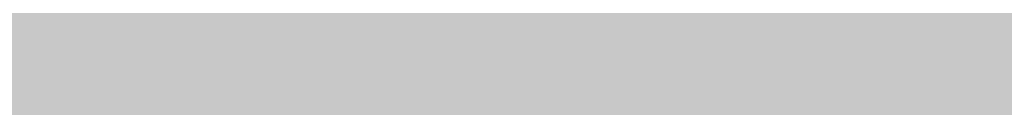
# Model space of a CAD drawing. Units: inches. Extents: x 2091 to 2899, y 967 to 2217.
# Tile 176 of 256: x 2203.151632 to 2203.161218, y 1152.2479 to 1152.248741. Entities that reach past the tile are written whole.
import ezdxf

# ---------------------------------------------------------------- set-up
doc = ezdxf.new("R2010")
doc.units = ezdxf.units.IN
doc.layers.add('A-WALL-PATT', color=141, linetype='Continuous', lineweight=13, true_color=0xadddf7)

msp = doc.modelspace()

# ---------------------------------------------------------------- hatches: boundary and pattern name
at = {"layer": 'A-WALL-PATT'}
h = msp.add_hatch(color=256, dxfattribs=at)
h.dxf.hatch_style = 1
h.paths.add_polyline_path([(2803.1436027, 2050.9190588), (2203.1436027, 2050.9190588), (2203.1436027, 1090.9190588), (2803.1436027, 1090.9190588)])
h.paths.add_polyline_path([(2635.7988501, 1147.5404649), (2674.5240524, 1147.5404649, 0.376086), (2678.5296653, 1152.8802017), (2678.5296653, 1159.5564734, 0.333335), (2674.524319, 1163.561846), (2674.524319, 1163.5618504), (2674.524319, 1192.9343904), (2635.8059707, 1192.9343904), (2597.0876225, 1192.9343904), (2597.0876225, 1163.561846, 0.333335), (2593.0822761, 1159.5564734), (2593.0822761, 1152.8802017, 0.376086), (2597.087889, 1147.5404649)], flags=0)
h.paths.add_polyline_path([(2436.0104329, 1278.2407784, 0.000483), (2435.9526433, 1278.215027, -0.001328), (2435.9356253, 1278.1116934, -0.001711), (2436.1164401, 1278.0407583, 0.002185)], flags=0)
h.paths.add_polyline_path([(2794.1436027, 1143.4190588), (2794.1436027, 1347.4190588), (2543.3701706, 1347.4190588), (2543.3701706, 1351.9190588), (2794.1436027, 1351.9190588), (2794.1436027, 1392.7135549), (2793.9473982, 1392.7135549), (2793.9473982, 1473.5368999), (2794.1436027, 1473.5368999), (2794.1436027, 1531.9190588), (2650.1436027, 1531.9190588), (2650.1436027, 1536.4190588), (2794.1436027, 1536.4190588), (2794.1436027, 1692.4190588), (2609.3756095, 1692.4190588), (2609.3756095, 1644.4190588), (2604.8756095, 1644.4190588), (2604.8756095, 1744.9190588), (2609.3756095, 1744.9190588), (2609.3756095, 1696.9190588), (2794.1436027, 1696.9190588), (2794.1436027, 1780.9190588), (2609.6436027, 1780.9190588), (2493.8756095, 1780.9190588), (2493.8756095, 1785.4190588), (2609.6436027, 1785.4190588), (2794.1436027, 1785.4190588), (2794.1436027, 1847.9388214), (2793.9512217, 1847.9388214), (2793.9512217, 1928.7621663), (2794.1436027, 1928.7621663), (2794.1436027, 1941.4190588), (2614.1436027, 1941.4190588), (2614.1436027, 1821.4190588), (2609.6436027, 1821.4190588), (2609.6436027, 1941.4190588), (2392.1436027, 1941.4190588), (2392.1436027, 1819.9190588), (2387.6436027, 1819.9190588), (2387.6436027, 1941.4190588), (2212.1436027, 1941.4190588), (2212.1436027, 1783.9190588), (2392.1436027, 1783.9190588), (2392.1436027, 1780.9190588), (2212.1436027, 1780.9190588), (2212.1436027, 1629.4190588), (2387.6436027, 1629.4190588), (2387.6436027, 1744.9190588), (2392.1436027, 1744.9190588), (2392.1436027, 1627.9190588), (2317.1436027, 1627.9190588), (2317.1436027, 1551.4190588), (2317.1436027, 1536.4190588), (2459.3835909, 1536.4190588), (2459.3835909, 1602.3964802), (2463.8835909, 1602.3964802), (2463.8835909, 1531.9190588), (2456.6436027, 1531.9190588), (2456.6436027, 1529.9190588), (2452.1436027, 1529.9190588), (2452.1436027, 1531.9190588), (2312.6436027, 1531.9190588), (2312.6436027, 1551.4190588), (2306.1436027, 1551.4190588), (2306.1436027, 1555.9190588), (2308.1436027, 1555.9190588), (2308.1436027, 1551.4190588), (2312.6436027, 1551.4190588), (2312.6436027, 1627.9190588), (2212.1436027, 1627.9190588), (2212.1436027, 1555.9190588), (2270.1436027, 1555.9190588), (2270.1436027, 1551.4190588), (2212.1436027, 1551.4190588), (2212.1436027, 1351.9190588), (2272.1436027, 1351.9190588), (2272.1436027, 1347.4190588), (2212.1436027, 1347.4190588), (2212.1436027, 1275.4190588), (2308.1436027, 1275.4190588), (2308.1436027, 1351.9190588), (2452.1436027, 1351.9190588), (2452.1436027, 1493.9190588), (2456.6436027, 1493.9190588), (2456.6436027, 1347.4190588), (2312.6436027, 1347.4190588), (2312.6436027, 1270.9190588), (2212.1436027, 1270.9190588), (2212.1436027, 1099.9190588), (2281.2375229, 1099.9190588), (2282.8710413, 1110.9138034), (2282.0083413, 1116.9966034), (2278.5577413, 1121.4204034), (2268.2056413, 1128.0562034), (2272.0876413, 1128.0562034), (2273.8129413, 1131.9270034), (2279.4203413, 1134.6919034), (2285.0278413, 1135.2449034), (2287.6158413, 1137.4568034), (2288.0471413, 1138.0098034), (2289.3411413, 1140.7747034), (2291.0665413, 1139.6687034), (2292.3605413, 1135.2449034), (2295.3798413, 1136.9038034), (2296.2425413, 1135.7979034), (2297.1052413, 1133.0330034), (2300.1246413, 1138.0098034), (2303.1439413, 1138.0098034), (2304.4379413, 1135.7979034), (2303.1439413, 1133.5860034), (2306.5946413, 1134.6919034), (2307.8887413, 1133.0330034), (2310.9080413, 1135.2449034), (2313.9274413, 1134.1389034), (2315.6268599, 1132.4271023), (2308.3200413, 1117.5496034), (2290.2038413, 1109.8079034), (2288.9098413, 1103.1721034), (2289.2723086, 1099.9190588), (2434.9182274, 1099.9190588), (2431.5932274, 1124.7880588), (2429.9302274, 1169.5530588), (2430.9271848, 1240.5196942), (2435.6589255, 1238.1861258), (2437.1352274, 1196.5540588), (2438.7982274, 1143.9730588), (2442.6782274, 1111.9980588), (2446.5582274, 1099.9190588), (2794.1436027, 1099.9190588), (2794.1436027, 1138.9190588), (2548.0324471, 1138.9190588), (2548.0324471, 1143.4190588), (2548.0324471, 1148.8190588), (2546.6684571, 1148.0315588), (2528.6856919, 1179.1786218, 0.256256), (2512.0324471, 1148.8190588), (2512.0324471, 1143.4190588), (2512.0324471, 1138.9190588), (2507.5324471, 1138.9190588), (2507.5324471, 1143.4190588), (2507.5324471, 1148.8190588, 0.256256), (2490.8792023, 1179.1786218), (2472.8964371, 1148.0315588), (2471.5324471, 1148.8190588), (2471.5324471, 1143.4190588), (2467.0324471, 1143.4190588), (2467.0324471, 1269.9457858, 0.039061), (2460.9099871, 1273.5800588), (2467.0324471, 1273.5800588), (2467.0324471, 1286.3253638, 0.014511), (2465.2161944, 1286.7619052), (2467.0324471, 1287.0525761), (2467.0324471, 1323.4190588), (2471.5324471, 1323.4190588), (2471.5324471, 1148.8190588), (2489.5324471, 1179.9959734), (2490.8964371, 1179.2084734), (2490.8792023, 1179.1786218, -0.256256), (2507.5324471, 1148.8190588), (2507.5324471, 1143.4190588), (2512.0324471, 1143.4190588), (2512.0324471, 1148.8190588, -0.256256), (2528.6856919, 1179.1786218), (2528.6684571, 1179.2084734), (2530.0324471, 1179.9959734), (2548.0324471, 1148.8190588), (2548.0324471, 1143.4190588)], flags=16)
h.paths.add_polyline_path([(2607.7685461, 1200.9450832), (2607.7685461, 1265.0306251), (2597.0876225, 1281.0520106), (2619.7845852, 1281.0520106), (2627.795278, 1337.1268598), (2635.7988501, 1337.1268598), (2643.8166634, 1337.1268598), (2651.8273562, 1281.0520106), (2674.524319, 1281.0520106), (2663.8433953, 1265.0306251), (2663.8433953, 1200.9450832), (2635.8059707, 1200.9450832)], flags=0)
edge = h.paths.add_edge_path(flags=0)
edge.add_ellipse((13303.8962153, 1272.9987247), major_axis=(-10595.3130399, 0.0000005), ratio=0.842303870086, start_angle=0.62823721906, end_angle=0.64655409989, ccw=False)
edge.add_ellipse((2711.7004495, 1156.8526781), major_axis=(2.2197691, 0), ratio=0.84230387, start_angle=111.5352435, end_angle=180.6282372, ccw=False)
edge.add_ellipse((13303.1562922, 1272.9987246), major_axis=(-10593.0263064, 0), ratio=0.842303869544, start_angle=0.52827147182, end_angle=0.64655409706, ccw=False)
edge.add_line((2710.7645961, 1175.3332951), (2710.1299858, 1175.3332951))
edge.add_ellipse((2710.1299858, 1176.5797752), major_axis=(1.4798461, 0), ratio=0.84230387, start_angle=180, end_angle=270, ccw=False)
edge.add_line((2708.6501397, 1176.5797752), (2708.6501397, 1200.7829144))
edge.add_ellipse((2710.1299858, 1200.7829144), major_axis=(1.4798461, 0), ratio=0.84230387, start_angle=90, end_angle=180, ccw=False)
edge.add_line((2710.1299858, 1202.0293944), (2710.4650752, 1202.0293944))
edge.add_ellipse((13303.1562922, 1272.9987246), major_axis=(-10593.0263064, 0), ratio=0.842303869544, start_angle=-0.09022908859, end_angle=0.38386677879, ccw=False)
edge.add_ellipse((2710.1299858, 1290.9270308), major_axis=(-1.4798461, 0), ratio=0.84230387, start_angle=0, end_angle=90, ccw=False)
edge.add_line((2708.6501397, 1290.9270308), (2708.6501397, 1315.13017))
edge.add_ellipse((2710.1299858, 1315.13017), major_axis=(-1.4798461, 0), ratio=0.84230387, start_angle=-90, end_angle=0, ccw=False)
edge.add_line((2710.1299858, 1316.3766501), (2710.7063141, 1316.3766501))
edge.add_ellipse((3238.4017202, 1296.2895655), major_axis=(528.2339998, 0), ratio=0.84230386954, start_angle=176.349572414, end_angle=177.820049686, ccw=False)
edge.add_ellipse((2775.0630432, 1071.4506962), major_axis=(313.3077613, 0), ratio=0.84230386954, start_angle=102.125965552, end_angle=103.780528989, ccw=False)
edge.add_ellipse((2775.0630432, 1078.3056979), major_axis=(-305.3028915, 0), ratio=0.84230386955, start_angle=-79.790461003, end_angle=-77.555372706, ccw=False)
edge.add_ellipse((2695.1417666, 1541.9753825), major_axis=(-250.9602162, 0), ratio=0.84230386954, start_angle=99.256566007, end_angle=102.554932644)
edge.add_line((2741.4103262, 1334.2142554), (2747.1325454, 1337.3784768))
edge.add_ellipse((2747.5386163, 1336.8574776), major_axis=(-0.739923, 0), ratio=0.84230387, start_angle=270, end_angle=307.9331305, ccw=False)
edge.add_ellipse((2747.5386163, 1336.8574776), major_axis=(-0.739923, 0), ratio=0.84230387, start_angle=232.0668695, end_angle=270, ccw=False)
edge.add_line((2747.9446872, 1337.3784768), (2753.6669064, 1334.2142554))
edge.add_ellipse((2799.935466, 1541.9753825), major_axis=(250.9602162, 0), ratio=0.84230386954, start_angle=257.445067356, end_angle=260.743433993)
edge.add_ellipse((2720.0141894, 1078.3056979), major_axis=(305.3028915, 0), ratio=0.84230386954, start_angle=77.555372707, end_angle=79.790461003, ccw=False)
edge.add_ellipse((2720.0141894, 1071.4506962), major_axis=(-313.3077613, 0), ratio=0.84230386954, start_angle=256.219471011, end_angle=257.874034448, ccw=False)
edge.add_ellipse((2256.6755124, 1296.2895655), major_axis=(-528.2339998, 0), ratio=0.84230386954, start_angle=182.179950314, end_angle=183.650427586, ccw=False)
edge.add_line((2784.3709184, 1316.3766501), (2784.9472468, 1316.3766501))
edge.add_ellipse((2784.9472468, 1315.13017), major_axis=(1.4798461, 0), ratio=0.84230387, start_angle=0, end_angle=90, ccw=False)
edge.add_line((2786.4270928, 1315.13017), (2786.4270928, 1290.9270308))
edge.add_ellipse((2784.9472468, 1290.9270308), major_axis=(1.4798461, 0), ratio=0.84230387, start_angle=270, end_angle=360, ccw=False)
edge.add_ellipse((-7808.0790596, 1272.9987246), major_axis=(10593.0263063, 0), ratio=0.842303869544, start_angle=-0.38386677879, end_angle=0.09022908859, ccw=False)
edge.add_line((2784.6121574, 1202.0293944), (2784.9472468, 1202.0293944))
edge.add_ellipse((2784.9472468, 1200.7829144), major_axis=(1.4798461, 0), ratio=0.84230387, start_angle=0, end_angle=90, ccw=False)
edge.add_line((2786.4270928, 1200.7829144), (2786.4270928, 1176.5797752))
edge.add_ellipse((2784.9472468, 1176.5797752), major_axis=(-1.4798461, 0), ratio=0.84230387, start_angle=90, end_angle=180, ccw=False)
edge.add_line((2784.9472468, 1175.3332951), (2784.3126365, 1175.3332951))
edge.add_ellipse((-7808.0790596, 1272.9987246), major_axis=(10593.0263063, 0), ratio=0.842303869544, start_angle=-0.61864319632, end_angle=-0.52827147182, ccw=False)
edge.add_ellipse((2783.3767831, 1156.8526781), major_axis=(-2.2197691, 0), ratio=0.84230387, start_angle=179.3717628, end_angle=248.4647566, ccw=False)
edge.add_ellipse((-7808.8189826, 1272.9987246), major_axis=(-10595.3130398, 0.0000036), ratio=0.842303865762, start_angle=179.3534459226, end_angle=179.37176280343, ccw=False)
edge.add_ellipse((2780.2973026, 1153.500793), major_axis=(-5.2464256, 0), ratio=0.84230387, start_angle=90, end_angle=179.3534459, ccw=False)
edge.add_line((2780.2973026, 1149.0817084), (2714.77993, 1149.0817084))
edge.add_ellipse((2714.77993, 1153.500793), major_axis=(5.2464256, 0), ratio=0.84230387, start_angle=180.6465541, end_angle=270, ccw=False)
edge = h.paths.add_edge_path(flags=0)
edge.add_line((2718.1873674, 1151.0078329), (2718.1873674, 1170.4723638))
edge.add_ellipse((2721.1470595, 1170.4723638), major_axis=(-2.9596921, 0), ratio=0.84230387, start_angle=-90, end_angle=0, ccw=False)
edge.add_line((2721.1470595, 1172.965324), (2773.9301731, 1172.965324))
edge.add_ellipse((2773.9301731, 1170.4723638), major_axis=(-2.9596921, 0), ratio=0.84230387, start_angle=180, end_angle=270, ccw=False)
edge.add_line((2776.8898652, 1170.4723638), (2776.8898652, 1151.0078329))
edge.add_line((2776.8898652, 1151.0078329), (2718.1873674, 1151.0078329))
edge = h.paths.add_edge_path(flags=0)
edge.add_line((2718.1873674, 1180.2341502), (2718.1873674, 1199.0578342))
edge.add_ellipse((2747.5386163, 1320.3986402), major_axis=(147.0179239, 0), ratio=0.84230386954, start_angle=256.40186531, end_angle=283.59813469)
edge.add_line((2776.8898652, 1199.0578342), (2776.8898652, 1180.2341502))
edge.add_ellipse((2747.5386163, 1301.5749562), major_axis=(147.0179239, 0), ratio=0.84230386954, start_angle=256.40186531, end_angle=283.59813469, ccw=False)
edge = h.paths.add_edge_path(flags=0)
edge.add_ellipse((13303.1562922, 1272.9987246), major_axis=(-10591.5464603, 0), ratio=0.842303869555, start_angle=0.05559431352, end_angle=0.37776419393, ccw=False)
edge.add_line((2711.6168595, 1262.7217103), (2715.6674076, 1249.4953957))
edge.add_ellipse((6413.8919626, 1241.691919), major_axis=(-3698.2361592, 0), ratio=0.842303869547, start_angle=-0.120897369, end_angle=0.3640763489)
edge.add_line((2715.7610383, 1218.1924547), (2711.9343065, 1203.167361))
edge = h.paths.add_edge_path(flags=0)
edge.add_line((2718.1873674, 1251.074566), (2716.0024854, 1267.4504351))
edge.add_ellipse((2742.1511746, 1202.1895399), major_axis=(81.7725845, 0), ratio=0.8423038695, start_angle=94.277420963, end_angle=111.834953797, ccw=False)
edge.add_line((2737.0097482, 1270.9306255), (2758.0674844, 1270.9306255))
edge.add_ellipse((2752.926058, 1202.1895399), major_axis=(81.7725845, 0), ratio=0.8423038695, start_angle=68.165046203, end_angle=85.722579037, ccw=False)
edge.add_line((2779.0747472, 1267.4504351), (2776.8898652, 1251.074566))
edge.add_ellipse((2750.3380588, 1187.8853558), major_axis=(79.5796641, 0), ratio=0.8423038695, start_angle=67.208085122, end_angle=85.129930403)
edge.add_line((2756.0346562, 1254.7436557), (2739.0425764, 1254.7436557))
edge.add_ellipse((2744.7391738, 1187.8853558), major_axis=(79.5796641, 0), ratio=0.8423038695, start_angle=94.870069597, end_angle=112.791914878)
edge = h.paths.add_edge_path(flags=0)
edge.add_line((2783.1429261, 1203.167361), (2779.3161943, 1218.1924547))
edge.add_ellipse((-918.81473, 1241.691919), major_axis=(3698.2361592, 0), ratio=0.842303869546, start_angle=-0.3640763489, end_angle=0.120897369)
edge.add_line((2779.409825, 1249.4953957), (2783.4603731, 1262.7217103))
edge.add_ellipse((-7808.0790596, 1272.9987246), major_axis=(-10591.5464603, 0), ratio=0.84230386954, start_angle=179.6222358061, end_angle=179.94440568651, ccw=False)
edge = h.paths.add_edge_path(flags=0)
edge.add_ellipse((2734.2008921, 1286.6904402), major_axis=(-0.3566086, 6.3400775), ratio=0.603833576, start_angle=89.00201428, end_angle=253.65740805, ccw=False)
edge.add_line((2730.3690013, 1286.5418057), (2730.3690013, 1301.3519803))
edge.add_line((2730.3690013, 1301.3519803), (2735.9133107, 1305.2148028))
edge.add_ellipse((2736.3849168, 1304.7345612), major_axis=(0.739923, 0), ratio=0.84230387, start_angle=90, end_angle=134.4802109, ccw=False)
edge.add_line((2736.3849168, 1305.3578013), (2738.0327829, 1305.3578013))
edge.add_line((2738.0327829, 1305.3578013), (2738.0327829, 1307.7079274))
edge.add_ellipse((2794.201642, 1307.7079274), major_axis=(56.168859, 0), ratio=0.8423038695, start_angle=150.5614304, end_angle=180, ccw=False)
edge.add_ellipse((2700.8755906, 1307.7079274), major_axis=(-56.168859, 0), ratio=0.8423038695, start_angle=180, end_angle=209.4385696, ccw=False)
edge.add_line((2757.0444497, 1307.7079274), (2757.0444497, 1305.3578013))
edge.add_line((2757.0444497, 1305.3578013), (2758.6923157, 1305.3578013))
edge.add_ellipse((2758.6923157, 1304.7345612), major_axis=(-0.739923, 0), ratio=0.84230387, start_angle=225.5197891, end_angle=270, ccw=False)
edge.add_line((2759.1639219, 1305.2148028), (2764.7082312, 1301.3519803))
edge.add_line((2764.7082312, 1301.3519803), (2764.7082312, 1286.5418057))
edge.add_ellipse((2760.8763405, 1286.6904402), major_axis=(0.3566086, 6.3400775), ratio=0.603833576, start_angle=106.34259195, end_angle=270.99798572, ccw=False)
edge.add_line((2757.0444497, 1285.7970896), (2757.0444497, 1307.7079274))
edge.add_ellipse((2700.8755906, 1307.7079274), major_axis=(-56.168859, 0), ratio=0.8423038695, start_angle=180, end_angle=209.4385696)
edge.add_ellipse((2794.201642, 1307.7079274), major_axis=(56.168859, 0), ratio=0.8423038695, start_angle=150.5614304, end_angle=180)
edge.add_line((2738.0327829, 1307.7079274), (2738.0327829, 1285.7970896))
h.paths.add_polyline_path([(2417.8122727, 1104.449704), (2413.4922727, 1102.529704), (2410.6122727, 1103.969704), (2409.1722727, 1106.369704), (2407.2522727, 1107.329704), (2406.2922727, 1109.729704), (2405.3322727, 1114.049704), (2405.3322727, 1117.889704), (2406.2922727, 1120.129704), (2407.2522727, 1119.809704), (2408.8483218, 1118.3276585), (2410.1739451, 1119.4241703), (2410.2112727, 1120.405704), (2411.0407305, 1121.4190541), (2410.6992727, 1119.858704), (2410.1739451, 1119.4241703), (2410.0884515, 1117.1761095), (2411.1328361, 1116.2063237), (2413.9722727, 1119.329704), (2416.8522727, 1120.769704), (2416.8697209, 1120.7987842), (2417.0350713, 1119.4051162), (2417.8962134, 1118.1433844), (2418.2922727, 1118.369704), (2419.5444467, 1120.0392692), (2419.3609153, 1118.387487), (2419.0321078, 1119.3561507), (2418.3989394, 1118.5119262), (2419.2522727, 1114.529704), (2418.7940909, 1107.1987949)], flags=0)
h.paths.add_polyline_path([(2508.8701706, 1347.4190588), (2508.3701706, 1347.4190588), (2508.3701706, 1351.9190588), (2508.8701706, 1351.9190588)], flags=0)
h.paths.add_polyline_path([(2473.3701706, 1347.4190588), (2472.3701706, 1347.4190588), (2467.8701706, 1347.4190588), (2467.8701706, 1455.4190588), (2472.3701706, 1455.4190588), (2472.3701706, 1352.4190588), (2473.3701706, 1352.4190588)], flags=0)
h.paths.add_polyline_path([(2352.106244, 1217.4461971), (2349.226244, 1218.8861971), (2347.786244, 1221.2861971), (2345.866244, 1222.2461971), (2344.906244, 1224.6461971), (2343.946244, 1228.9661971), (2343.946244, 1232.8061971), (2344.906244, 1235.0461971), (2345.866244, 1234.7261971), (2347.4622931, 1233.2441515), (2348.7879164, 1234.3406634), (2348.825244, 1235.3221971), (2349.6547018, 1236.3355471), (2349.313244, 1234.7751971), (2348.7879164, 1234.3406634), (2348.7024228, 1232.0926025), (2349.7468074, 1231.1228168), (2352.586244, 1234.2461971), (2355.466244, 1235.6861971), (2355.4836921, 1235.7152773), (2355.6490426, 1234.3216093), (2356.5101846, 1233.0598774), (2356.906244, 1233.2861971), (2358.1584179, 1234.9557623), (2357.9748866, 1233.3039801), (2357.6460791, 1234.2726438), (2357.0129107, 1233.4284193), (2357.866244, 1229.4461971), (2357.4080622, 1222.115288), (2356.426244, 1219.3661971)], flags=0)
h.paths.add_polyline_path([(2348.2967999, 1112.2244204), (2347.0137999, 1112.3104204), (2345.5297999, 1114.1274204), (2345.7317999, 1115.8584204), (2346.8117999, 1116.9824204), (2346.8117999, 1114.6464204), (2345.8667999, 1114.2144204), (2346.8797999, 1114.3004204)], flags=0)
h.paths.add_polyline_path([(2347.0137999, 1110.9264204), (2346.2717999, 1110.4934204), (2346.6097999, 1111.1864204)], flags=0)
h.paths.add_polyline_path([(2345.8667999, 1118.1944204), (2345.5297999, 1117.3294204), (2343.7077999, 1118.0214204), (2344.3827999, 1118.6264204)], flags=0)
h.paths.add_polyline_path([(2346.6767999, 1109.2824204), (2346.0697999, 1108.0714204), (2345.8667999, 1110.0614204)], flags=0)
h.paths.add_polyline_path([(2345.0567999, 1119.7514204), (2343.6397999, 1119.7514204), (2343.9777999, 1121.1354204)], flags=0)
h.paths.add_polyline_path([(2345.2597999, 1116.5504204), (2345.1247999, 1115.8584204), (2344.9217999, 1115.6854204), (2344.7197999, 1116.3774204)], flags=0)
h.paths.add_polyline_path([(2345.6647999, 1112.3104204), (2345.4617999, 1111.5324204), (2344.0447999, 1111.9644204), (2344.6517999, 1112.5704204)], flags=0)
h.paths.add_polyline_path([(2345.1917999, 1113.3494204), (2344.4497999, 1113.8684204), (2344.7197999, 1114.3874204)], flags=0)
h.paths.add_polyline_path([(2344.6517999, 1116.8094204), (2344.1797999, 1115.6854204), (2344.6517999, 1115.3394204), (2343.9097999, 1114.9064204), (2343.0327999, 1115.9444204), (2343.6397999, 1116.4634204)], flags=0)
h.paths.add_polyline_path([(2345.8667999, 1106.6864204), (2344.9897999, 1105.5624204), (2344.5167999, 1106.6004204)], flags=0)
h.paths.add_polyline_path([(2344.8547999, 1110.0614204), (2344.5167999, 1109.2824204), (2344.1127999, 1109.7154204)], flags=0)
h.paths.add_polyline_path([(2344.0447999, 1113.5224204), (2343.4377999, 1113.0894204), (2342.7627999, 1113.9544204)], flags=0)
h.paths.add_polyline_path([(2344.3147999, 1111.0124204), (2342.9647999, 1110.3204204), (2342.9647999, 1111.0994204)], flags=0)
h.paths.add_polyline_path([(2345.1247999, 1104.6974204), (2344.5847999, 1103.7454204), (2344.4497999, 1104.2644204)], flags=0)
h.paths.add_polyline_path([(2342.8297999, 1121.2224204), (2341.7497999, 1120.5304204), (2340.5357999, 1121.0494204), (2340.1307999, 1121.8284204), (2340.6707999, 1122.9524204), (2341.1427999, 1121.8284204), (2341.6147999, 1122.0014204)], flags=0)
h.paths.add_polyline_path([(2342.9647999, 1119.7514204), (2343.0327999, 1118.4534204), (2342.0877999, 1118.0214204), (2342.0197999, 1119.4914204)], flags=0)
h.paths.add_polyline_path([(2342.6947999, 1116.8964204), (2341.9527999, 1116.6364204), (2342.0197999, 1117.3294204)], flags=0)
h.paths.add_polyline_path([(2343.0327999, 1112.2244204), (2342.0197999, 1111.7914204), (2341.5477999, 1112.2244204), (2342.3577999, 1113.3494204)], flags=0)
h.paths.add_polyline_path([(2343.7747999, 1104.4374204), (2342.6277999, 1102.8804204), (2342.6947999, 1104.6104204), (2343.4377999, 1105.1294204)], flags=0)
h.paths.add_polyline_path([(2342.0197999, 1115.0794204), (2340.8057999, 1115.5124204), (2340.9407999, 1116.3774204)], flags=0)
h.paths.add_polyline_path([(2341.4807999, 1120.0974204), (2341.4807999, 1119.4054204), (2341.0757999, 1119.5784204), (2341.1427999, 1120.0974204)], flags=0)
h.paths.add_polyline_path([(2341.8177999, 1114.4734204), (2340.9407999, 1113.0894204), (2340.8057999, 1114.5604204)], flags=0)
h.paths.add_polyline_path([(2341.1427999, 1118.5404204), (2340.9407999, 1116.9824204), (2339.0507999, 1117.6754204), (2339.0507999, 1118.6264204)], flags=0)
h.paths.add_polyline_path([(2342.6947999, 1101.6684204), (2341.9527999, 1101.8414204), (2342.5597999, 1102.3614204)], flags=0)
h.paths.add_polyline_path([(2340.3327999, 1119.6654204), (2338.4437999, 1119.5784204), (2337.9037999, 1120.3574204), (2339.6577999, 1120.6164204)], flags=0)
h.paths.add_polyline_path([(2340.3327999, 1115.3394204), (2340.0627999, 1113.6954204), (2339.3877999, 1115.3394204)], flags=0)
h.paths.add_polyline_path([(2341.8177999, 1103.8314204), (2341.5477999, 1102.8804204), (2341.1427999, 1103.6584204)], flags=0)
h.paths.add_polyline_path([(2339.0507999, 1122.8664204), (2337.2957999, 1121.8284204), (2337.0937999, 1123.1254204), (2337.7687999, 1123.8184204)], flags=0)
h.paths.add_polyline_path([(2339.1177999, 1121.7414204), (2338.8477999, 1121.2224204), (2338.1737999, 1121.0494204), (2338.3757999, 1121.5684204)], flags=0)
h.paths.add_polyline_path([(2339.1857999, 1119.3194204), (2338.6457999, 1118.7134204), (2338.2407999, 1118.1074204), (2338.2407999, 1118.8864204)], flags=0)
h.paths.add_polyline_path([(2341.1427999, 1101.9284204), (2340.6027999, 1101.2364204), (2340.0627999, 1101.8414204), (2340.6027999, 1102.3614204)], flags=0)
h.paths.add_polyline_path([(2337.6337999, 1117.7614204), (2336.6207999, 1118.2804204), (2337.2957999, 1118.9724204)], flags=0)
h.paths.add_polyline_path([(2336.8237999, 1119.5784204), (2334.7987999, 1118.9724204), (2335.2037999, 1120.3574204), (2336.5537999, 1120.8764204)], flags=0)
h.paths.add_polyline_path([(2339.1177999, 1100.4574204), (2337.3637999, 1100.5434204), (2336.7557999, 1101.2364204)], flags=0)
h.paths.add_polyline_path([(2336.3507999, 1122.4334204), (2336.0137999, 1121.9144204), (2334.9337999, 1122.4334204), (2334.5287999, 1123.4714204), (2335.7437999, 1122.7794204)], flags=0)
h.paths.add_polyline_path([(2334.7317999, 1120.8764204), (2334.2587999, 1120.3574204), (2334.0567999, 1120.7894204), (2334.5967999, 1121.3084204)], flags=0)
h.paths.add_polyline_path([(2334.4617999, 1122.1744204), (2332.5717999, 1121.3084204), (2331.3567999, 1122.1744204), (2332.0997999, 1122.8664204)], flags=0)
h.paths.add_polyline_path([(2334.2587999, 1118.5404204), (2333.3817999, 1118.4534204), (2333.6517999, 1119.3194204)], flags=0)
h.paths.add_polyline_path([(2335.5417999, 1102.2744204), (2334.1917999, 1102.6204204), (2335.2717999, 1103.3124204)], flags=0)
h.paths.add_polyline_path([(2332.7067999, 1119.6654204), (2331.6947999, 1120.4434204), (2332.5047999, 1120.7894204)], flags=0)
h.paths.add_polyline_path([(2334.7317999, 1101.1494204), (2333.5167999, 1101.5824204), (2333.9887999, 1101.7554204)], flags=0)
h.paths.add_polyline_path([(2332.6397999, 1116.6364204), (2331.0867999, 1116.2904204), (2331.9647999, 1118.1944204)], flags=0)
h.paths.add_polyline_path([(2330.7497999, 1121.5684204), (2330.2767999, 1120.2704204), (2328.5227999, 1119.3194204), (2328.9947999, 1121.0494204)], flags=0)
h.paths.add_polyline_path([(2330.7497999, 1118.6264204), (2330.0077999, 1117.5024204), (2329.8727999, 1118.0214204)], flags=0)
h.paths.add_polyline_path([(2332.0997999, 1102.3614204), (2330.5467999, 1102.0144204), (2331.6947999, 1102.9664204)], flags=0)
h.paths.add_polyline_path([(2329.5347999, 1113.6084204), (2329.0627999, 1112.3104204), (2328.5897999, 1113.3494204)], flags=0)
h.paths.add_polyline_path([(2328.3877999, 1117.8484204), (2327.5097999, 1116.5504204), (2327.1727999, 1117.7614204)], flags=0)
h.paths.add_polyline_path([(2329.7377999, 1106.5134204), (2329.5347999, 1105.3024204), (2328.2527999, 1106.0814204)], flags=0)
h.paths.add_polyline_path([(2328.6577999, 1114.3874204), (2328.0497999, 1114.1274204), (2328.3197999, 1114.9064204)], flags=0)
h.paths.add_polyline_path([(2328.3197999, 1112.2244204), (2327.1057999, 1112.1374204), (2326.7007999, 1112.6564204)], flags=0)
h.paths.add_polyline_path([(2326.9027999, 1115.2524204), (2326.7007999, 1114.1274204), (2325.2157999, 1113.6084204), (2326.0927999, 1115.3394204)], flags=0)
h.paths.add_polyline_path([(2326.6327999, 1108.3304204), (2326.0927999, 1107.3794204), (2325.8907999, 1108.5034204), (2326.4977999, 1109.1094204)], flags=0)
h.paths.add_polyline_path([(2615.1436027, 1531.9190588), (2609.6436027, 1531.9190588), (2609.6436027, 1620.4190588), (2614.1436027, 1620.4190588), (2614.1436027, 1536.4190588), (2615.1436027, 1536.4190588)], flags=0)
h.paths.add_polyline_path([(2545.1436027, 1563.4190588), (2464.1436027, 1563.4190588), (2464.1436027, 1632.4190588), (2509.1436027, 1632.4190588), (2509.1436027, 1627.9190588), (2509.1436027, 1603.9190588), (2468.6436027, 1603.9190588), (2468.6436027, 1567.9190588), (2540.6436027, 1567.9190588), (2540.6436027, 1591.9190588), (2545.1436027, 1591.9190588)], flags=0)
h.paths.add_polyline_path([(2388.9690483, 1549.985735), (2357.4341811, 1549.985735), (2357.4341811, 1623.3607783), (2399.3627772, 1623.3607783), (2435.6894654, 1623.3607783), (2435.5925469, 1602.5592734), (2435.5925469, 1602.3964802), (2388.9690483, 1602.3964802)], flags=0)
h.paths.add_polyline_path([(2388.8806282, 1555.8091511), (2374.9044295, 1555.8091511), (2374.9044295, 1600.5715641), (2374.9044295, 1615.4576454), (2406.3508766, 1615.4576454), (2406.3508766, 1618.9394309), (2412.1742927, 1615.4576454), (2406.3508766, 1611.9758599), (2406.3508766, 1615.4576454), (2388.8806282, 1615.4576454)], flags=0)
h.paths.add_polyline_path([(2568.8756095, 1644.4190588), (2453.3756095, 1644.4190588), (2453.3756095, 1785.4190588), (2457.8756095, 1785.4190588), (2457.8756095, 1648.9190588), (2568.8756095, 1648.9190588)], flags=0)
h.paths.add_polyline_path([(2212.1436027, 1945.9190588), (2212.1436027, 2041.9190588), (2794.1436027, 2041.9190588), (2794.1436027, 1945.9190588)], flags=16)
h.paths.add_polyline_path([(2271.0827276, 1964.3172377), (2776.852968, 1964.3172377), (2776.852968, 2037.1696226), (2271.0827276, 2037.1696226)], flags=8)
h.paths.add_polyline_path([(2380.6492852, 1536.8241435), (2461.0408087, 1536.8241435), (2461.0408087, 1554.6525871), (2380.6492852, 1554.6525871)], flags=8)
h.paths.add_polyline_path([(2240.7557092, 1609.7254508), (2309.1858294, 1609.7254508), (2309.1858294, 1617.6982037), (2240.7557092, 1617.6982037)], flags=8)
h.paths.add_polyline_path([(2212.6772554, 1313.5041021), (2282.5915203, 1313.5041021), (2282.5915203, 1322.7452389), (2212.6772554, 1322.7452389)], flags=8)
h.paths.add_polyline_path([(2457.111976, 1114.778574), (2558.4815807, 1114.778574), (2558.4815807, 1142.2196823), (2457.111976, 1142.2196823)], flags=8)
h.paths.add_polyline_path([(2473.4423372, 1273.0100672), (2604.6412257, 1273.0100672), (2604.6412257, 1318.3469349), (2473.4423372, 1318.3469349)], flags=8)
h.paths.add_polyline_path([(2638.8763024, 1626.9774316), (2684.2503675, 1627.9767377), (2684.0384825, 1637.5974944), (2638.6644174, 1636.5981884)], flags=8)
h.paths.add_polyline_path([(2537.5905538, 1453.7934466), (2628.3895472, 1453.7934466), (2628.3895472, 1475.3448114), (2537.5905538, 1475.3448114)], flags=8)
h.paths.add_polyline_path([(2504.1376376, 1714.6323972), (2554.6471875, 1714.6323972), (2554.6471875, 1730.2377115), (2504.1376376, 1730.2377115)], flags=8)
h.paths.add_polyline_path([(2487.5011806, 1575.6518716), (2535.0971214, 1575.6518716), (2535.0971214, 1598.3776456), (2487.5011806, 1598.3776456)], flags=8)
h.paths.add_polyline_path([(2709.0994004, 1735.7102784), (2740.0166009, 1735.7102784), (2740.0166009, 1749.9376406), (2709.0994004, 1749.9376406)], flags=8)
h.paths.add_polyline_path([(2442.4384239, 1792.1716575), (2564.7288353, 1792.1716575), (2564.7288353, 1842.0001626), (2442.4384239, 1842.0001626)], flags=8)
h.paths.add_polyline_path([(2655.8158012, 1809.6440763), (2789.5201425, 1806.6937963), (2790.0849768, 1832.2916379), (2656.3806355, 1835.2419179)], flags=8)
h.paths.add_polyline_path([(2234.8426972, 1797.7201432), (2368.5928512, 1794.7688523), (2369.1607182, 1820.504132), (2235.4105642, 1823.4554229)], flags=8)
h.paths.add_polyline_path([(2245.1384659, 1644.0063348), (2398.4277329, 1640.6238997), (2398.9948417, 1666.3248199), (2245.7055747, 1669.7072549)], flags=8)
h.paths.add_polyline_path([(2306.1428474, 1431.1685186), (2413.7683138, 1428.7936873), (2414.3331481, 1454.3915289), (2306.7076817, 1456.7663602)], flags=8)
h.paths.add_polyline_path([(2306.834582, 1458.2331447), (2393.3804836, 1456.3234487), (2393.9328082, 1481.3543583), (2307.3869066, 1483.2640542)], flags=8)

doc.saveas('drawing.dxf')
